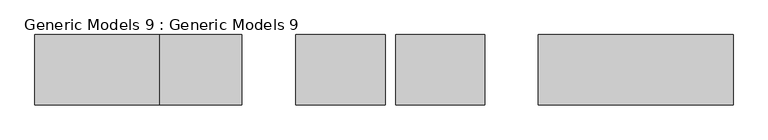
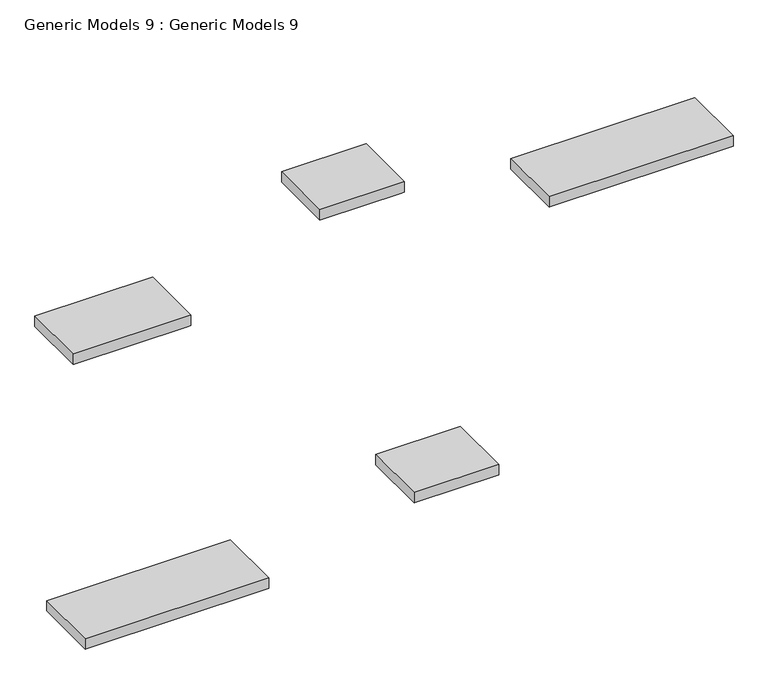
"""IFC4 building model written with IfcOpenShell, lengths in millimetres: proxy geometry, Generic Models 9 : Generic Models 9."""

from ifc_helpers import new_model, si_unit, frame, origin, place, context, project, spatial, polyline, outline, extrude, source, transform, mapped, element, save


def generic_models_9_generic_models_9_de2daabc(model_context):
    return source(origin(), model_context, "Body", "SweptSolid", [
        extrude(outline(polyline([(5238.75, -3294.2019453), (5238.75, -3268.8019453), (5238.75, -1630.5019453), (5238.75, -1605.1019453), (5340.35, -1605.1019453), (5340.35, -3294.2019453), (5238.75, -3294.2019453)])), frame((0.0, 16519.6444012, 0.0), z_axis=(0.0, 1.0, 0.0), x_axis=(0.0, 0.0, 1.0)), (0.0, 0.0, 1.0), 609.6),
        extrude(outline(polyline([(5848.35, -5396.0519453), (5848.35, -5370.6519453), (5848.35, -4646.7519453), (5848.35, -4621.3519453), (5949.95, -4621.3519453), (5949.95, -5396.0519453), (5848.35, -5396.0519453)])), frame((0.0, 16519.6444012, 0.0), z_axis=(0.0, 1.0, 0.0), x_axis=(0.0, 0.0, 1.0)), (0.0, 0.0, 1.0), 609.6),
        extrude(outline(polyline([(5238.75, -7659.8269453), (5238.75, -7634.4269453), (5238.75, -6605.7269453), (5238.75, -6580.3269453), (5340.35, -6580.3269453), (5340.35, -7659.8269453), (5238.75, -7659.8269453)])), frame((0.0, 16519.6444012, 0.0), z_axis=(0.0, 1.0, 0.0), x_axis=(0.0, 0.0, 1.0)), (0.0, 0.0, 1.0), 609.6),
        extrude(outline(polyline([(2800.35, -4532.4519453), (2800.35, -4507.0519453), (2800.35, -3783.1519453), (2800.35, -3757.7519453), (2901.95, -3757.7519453), (2901.95, -4532.4519453), (2800.35, -4532.4519453)])), frame((0.0, 16519.6444012, 0.0), z_axis=(0.0, 1.0, 0.0), x_axis=(0.0, 0.0, 1.0)), (0.0, 0.0, 1.0), 609.6),
        extrude(outline(polyline([(2438.0198917, -7551.1187626), (2438.0198917, -7525.7187626), (2438.0198917, -5891.3519453), (2438.0198917, -5865.9519453), (2539.6198917, -5865.9519453), (2539.6198917, -7551.1187626), (2438.0198917, -7551.1187626)])), frame((0.0, 16519.6444012, 0.0), z_axis=(0.0, 1.0, 0.0), x_axis=(0.0, 0.0, 1.0)), (0.0, 0.0, 1.0), 609.6),
    ])


if __name__ == "__main__":
    model = new_model("IFC4")
    model_context = context("Model", 3, world=origin())
    ifc_project = project(units=[si_unit("LENGTHUNIT", "METRE", prefix="MILLI")], contexts=[model_context])
    site = spatial("IfcSite", under=ifc_project)
    building = spatial("IfcBuilding", under=site)
    placement = place(None, origin())
    generic_models_9_generic_models_9_shape = generic_models_9_generic_models_9_de2daabc(model_context)
    element("IfcBuildingElementProxy", 1, Name="Generic Models 9 : Generic Models 9", ObjectType="Generic Models 9 : Generic Models 9", at=placement, inside=building, context=model_context, shape_type="MappedRepresentation", body=[
        mapped(generic_models_9_generic_models_9_shape, transform((0.0, 0.0, 0.0), x_axis=(1.0, 0.0, 0.0), y_axis=(0.0, 1.0, 0.0), z_axis=(0.0, 0.0, 1.0))),
    ])
    save(model, "model.ifc")
